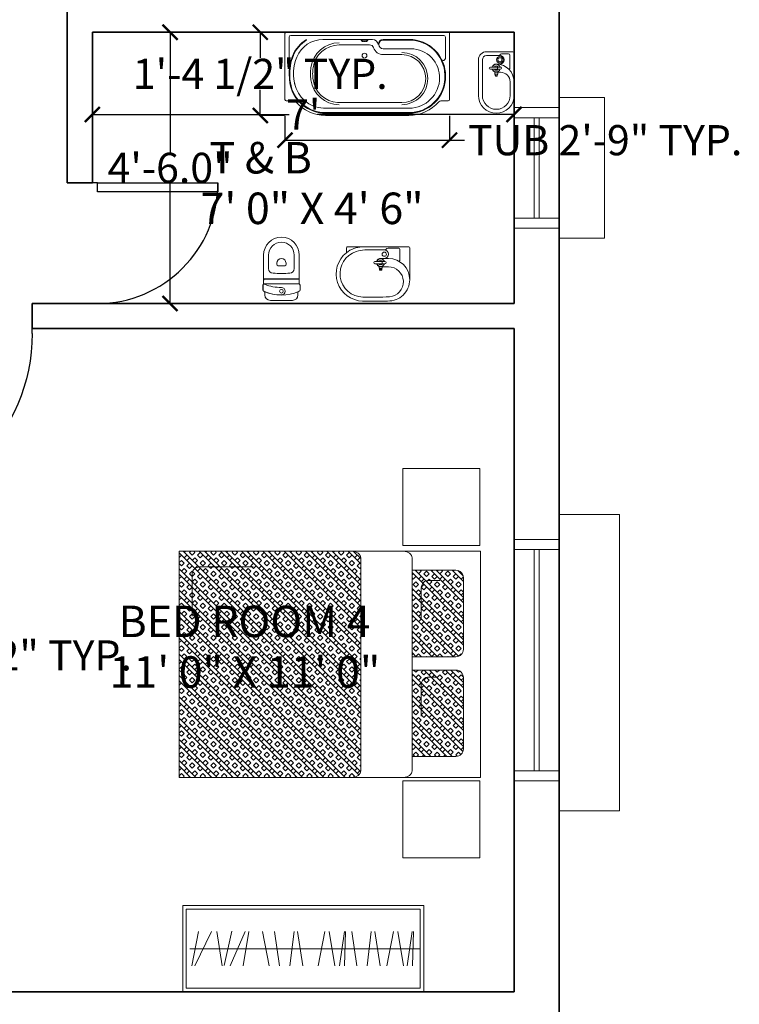
# Model space of a CAD drawing. Units: inches. Extents: x 844 to 2234, y 346 to 1084.
# Tile 91 of 93: x 2069 to 2212, y 632 to 828. Entities that reach past the tile are written whole.
import ezdxf

# ---------------------------------------------------------------- set-up
doc = ezdxf.new("R2010")
doc.units = ezdxf.units.IN
doc.header["$MEASUREMENT"] = 0
for name, color, linetype, lineweight in [('A-ANNO-DIMS', 2, 'Continuous', 18), ('A-AREA-IDEN', 7, 'Continuous', 18), ('A-FLOR-FIXT', 8, 'Continuous', 18), ('A-WALL', 7, 'Continuous', 35), ('beds', 130, 'Continuous', 18), ('doors', 170, 'Continuous', 25), ('furniture', 8, 'Continuous', 18), ('windows', 1, 'Continuous', 18)]:
    doc.layers.add(name, color=color, linetype=linetype, lineweight=lineweight)
doc.styles.get("Standard").update_dxf_attribs({"font": 'arial.ttf'})
doc.dimstyles.get("Standard").update_dxf_attribs({"dimtxt": 6, "dimasz": 3, "dimexe": 0.18, "dimexo": 0.0625, "dimgap": 0.09, "dimtad": 0, "dimtih": 1, "dimtoh": 1, "dimdec": 1, "dimzin": 0, "dimdsep": 46, "dimlunit": 3, "dimtxsty": 'Standard', "dimblk": 'ARCHTICK', "dimcen": 0.09, "dimadec": 0, "dimazin": 0, "dimtfac": 1, "dimtdec": 1, "dimtofl": 0, "dimtmove": 0, "dimatfit": 3, "dimfxl": 1, "dimtolj": 1, "dimtzin": 0, "dimarcsym": 0})
pattern_1 = [(135, (-1377.70473, -125.71507), (-0.070710678, -0.070710678), []), (135, (-1377.68705, -125.69739), (-0.070710678, -0.070710678), []), (45, (-1377.70473, -125.71507), (-0.070710678, 0.070710678), [-0.025, 0.025]), (45, (-1377.72241, -125.69739), (-0.070710678, 0.070710678), [-0.025, 0.025]), (45, (-1377.74009, -125.67972), (-0.070710678, 0.070710678), [0.025, -0.025]), (45, (-1377.75776, -125.66204), (-0.070710678, 0.070710678), [0.025, -0.025]), (135, (-1377.66938, -125.67972), (-0.070710678, -0.070710678), [0.025, -0.025]), (135, (-1377.6517, -125.66204), (-0.070710678, -0.070710678), [0.025, -0.025])]

# ---------------------------------------------------------------- blocks, each defined once
blk = doc.blocks.new('*U2')
for p, q in [((0, 0), (0, -6)), ((36, 0), (36, -6))]:
    blk.add_line(p, q)
blk.add_lwpolyline([(0, 0), (0, 36), (1.75, 36), (1.75, 0)], close=True)
blk.add_arc((0, 0), 36, 0, 90)
blk = doc.blocks.new('*U4')
for p, q in [((0, 0), (0, -6)), ((24, 0), (24, -6))]:
    blk.add_line(p, q)
blk.add_lwpolyline([(0, 0), (0, 24), (1.75, 24), (1.75, 0)], close=True)
blk.add_arc((0, 0), 24, 0, 90)
blk = doc.blocks.new('MAT-P10')
h = blk.add_hatch()
h.set_pattern_fill('BOX', color=256, scale=0.1, angle=45, style=0)
h.set_pattern_definition(pattern_1)
h.paths.add_polyline_path([(-0.1565, 1.4605), (0.417, 1.4605), (0.417, 1.7513, 0.414214), (0.367, 1.8013), (-0.1065, 1.8013, 0.414214), (-0.1565, 1.7513)])
h.paths.add_polyline_path([(0.5052, 1.4604), (1.0792, 1.4604), (1.0792, 1.7513, 0.414214), (1.0292, 1.8013), (0.5552, 1.8013, 0.414214), (0.5052, 1.7513)])
h = blk.add_hatch()
h.set_pattern_fill('BOX', color=256, scale=0.1, angle=45, style=0)
h.set_pattern_definition(pattern_1)
edge = h.paths.add_edge_path()
edge.add_line((1.2049, -0.085), (1.2049, 1.0625))
edge.add_ellipse((1.1608, 1.0627), major_axis=(0, 0.0568), ratio=0.776379, start_angle=270, end_angle=360)
edge.add_line((1.1608, 1.1195), (-0.251, 1.1195))
edge.add_ellipse((-0.251, 1.0627), major_axis=(0, 0.0568), ratio=0.776379, start_angle=0, end_angle=88.13958)
edge.add_line((-0.2951, 1.0641), (-0.2951, -0.085))
edge.add_line((-0.2951, -0.085), (1.2049, -0.085))
for p, q in [((-0.251, 1.4605), (1.1608, 1.4604)), ((-0.251, 1.1195), (1.1608, 1.1195)), ((1.1017, 0.406), (1.1017, 0.0572)), ((1.0576, 0.0004), (0.7754, 0.0004))]:
    blk.add_line(p, q)
for points in [[(-0.8301, 1.9091), (-0.3191, 1.9091), (-0.3191, 1.3981), (-0.8301, 1.3981)], [(1.2049, -0.085), (-0.2951, -0.085), (-0.2951, 1.9151), (1.2049, 1.915)], [(1.2441, 1.9091), (1.755, 1.9091), (1.755, 1.3981), (1.2441, 1.3981)]]:
    blk.add_lwpolyline(points, close=True)
for points in [[(0.417, 1.4604), (0.417, 1.7513, 0.414214), (0.367, 1.8013), (-0.1065, 1.8013, 0.414214), (-0.1565, 1.7513), (-0.1565, 1.4604)], [(1.0792, 1.4603), (1.0792, 1.7513, 0.414214), (1.0292, 1.8013), (0.5552, 1.8013, 0.414214), (0.5052, 1.7513), (0.5052, 1.4604)], [(1.0117, 1.6438), (1.0117, 1.5715, -0.414214), (0.9617, 1.5215), (0.7528, 1.5215)], [(0.3702, 1.6242), (0.3702, 1.5715, -0.414214), (0.3202, 1.5215), (0.1113, 1.5215)]]:
    blk.add_lwpolyline(points, format="xyb")
at = {"extrusion": (0, 0, -1)}
for centre, start_param, end_param in [((-0.251, 1.4036), 4.712389, 6.283185), ((1.1608, 1.4036), 0, 1.570796), ((-0.251, 1.0627), 4.712389, 6.283185), ((1.1608, 1.0627), 0, 1.570796), ((1.0576, 0.0572), 1.570796, 3.141593), ((1.0576, 0.0572), 1.570796, 3.141593)]:
    blk.add_ellipse(centre, major_axis=(0, 0.0568), ratio=0.776379, start_param=start_param, end_param=end_param, dxfattribs=at)
blk = doc.blocks.new('A$C7A17768A')
for p, q in [((-2.8, 0), (0, 0)), ((-2.8, -1), (-2.8, 0)), ((0, -1), (0, 0)), ((-2.76, -0.04), (-0.04, -0.04)), ((-2.76, -0.96), (-2.76, -0.04)), ((-0.04, -0.96), (-0.04, -0.04)), ((-2.617, -0.3), (-2.694, -0.7)), ((-2.66, -0.7), (-2.466, -0.3)), ((-2.403, -0.3), (-2.342, -0.7)), ((-2.229, -0.296), (-2.317, -0.696)), ((-2.074, -0.3), (-2.25, -0.7)), ((-2.096, -0.7), (-2.033, -0.3)), ((-1.875, -0.3), (-1.796, -0.7)), ((-1.732, -0.3), (-1.675, -0.7)), ((-1.555, -0.7), (-1.507, -0.3)), ((-1.467, -0.3), (-1.403, -0.7)), ((-1.227, -0.7), (-1.151, -0.3)), ((-1.098, -0.3), (-1.034, -0.7)), ((-0.98, -0.7), (-0.921, -0.3)), ((-0.908, -0.3), (-0.919, -0.7)), ((-0.834, -0.3), (-0.777, -0.7)), ((-0.657, -0.7), (-0.61, -0.3)), ((-0.57, -0.3), (-0.505, -0.7)), ((-0.429, -0.7), (-0.353, -0.3)), ((-0.301, -0.3), (-0.237, -0.7)), ((-0.192, -0.7), (-0.133, -0.3)), ((-0.12, -0.3), (-0.131, -0.7)), ((-0.04, -0.5), (-2.716, -0.5)), ((-2.8, -1), (0, -1)), ((-2.76, -0.96), (-0.04, -0.96))]:
    blk.add_line(p, q)
blk = doc.blocks.new('2SABICO')
at = {"color": 0, "linetype": 'ByBlock'}
for p, q in [((0.478, 0.195), (0.089, 0.195)), ((0.478, 0.152), (0.089, 0.152)), ((0, 0.106), (0, 0)), ((0, 0), (0, -0.18)), ((0.043, -0.039), (0.043, 0.106)), ((0.135, 0), (0.135, -0.003)), ((0.168, 0.064), (0.168, -0.015)), ((0.192, 0.064), (0.192, -0.015)), ((0.221, 0.012), (0.222, 0.012)), ((0.223, 0.016), (0.223, -0.016)), ((0.224, 0.017), (0.245, 0.017)), ((0.246, 0.016), (0.246, -0.016)), ((0.25, 0.014), (0.246, 0.014)), ((0.26, 0.01), (0.268, 0.01)), ((0.268, -0.01), (0.268, 0.01)), ((0.268, 0.01), (0.269, 0.009)), ((0.269, -0.009), (0.269, 0.009)), ((0.023, -0.057), (0.023, -0.135)), ((0.135, 0), (0.135, -0.039)), ((0.168, -0.015), (0.192, -0.015)), ((0.168, -0.015), (0.168, -0.046)), ((0.192, -0.015), (0.192, -0.046)), ((0.221, -0.012), (0.222, -0.012)), ((0.224, -0.017), (0.245, -0.017)), ((0.225, -0.017), (0.225, -0.047)), ((0.25, -0.014), (0.246, -0.014)), ((0.26, -0.01), (0.268, -0.01)), ((0.268, -0.01), (0.269, -0.009)), ((0.015, -0.195), (0.478, -0.195)), ((0.038, -0.15), (0.179, -0.15)), ((0.33, -0.152), (0.478, -0.152))]:
    blk.add_line(p, q, dxfattribs=at)
for radius in [0.035, 0.023]:
    blk.add_circle((0.089, -0.039), radius, dxfattribs=at)
for centre, radius, start, end in [((0.089, 0.106), 0.089, 90, 180), ((0.089, 0.106), 0.046, 90, 180), ((0.478, 0), 0.195, 270, 90), ((0.478, 0), 0.152, 270, 90), ((0.18, 0), 0.045, 105.6643, 180), ((0.18, 0), 0.042, 106.8152, 252.6853), ((0.18, 0), 0.0235, 121.1327, 237.8651), ((0.18, 0.064), 0.0121, 0, 180), ((0.18, 0), 0.045, 17.0576, 74.3357), ((0.18, 0), 0.042, 287.3147, 73.1848), ((0.18, 0), 0.0235, 302.1349, 58.8673), ((0.221, 0.013), 0.001, 197.9471, 270), ((0.222, 0.013), 0.001, 270, 0), ((0.224, 0.016), 0.001, 90, 180), ((0.245, 0.016), 0.001, 0, 90), ((0.25, 0), 0.0143, 270, 90), ((0.041, -0.057), 0.018, 99.5941, 180), ((0.037, -0.033), 0.006, 279.5941, 0), ((0.089, -0.039), 0.046, 180, 360), ((0.326, -0.003), 0.191, 180, 270), ((0.18, -0.046), 0.0125, 180, 0), ((0.221, -0.013), 0.001, 90, 162.0529), ((0.222, -0.013), 0.001, 0, 90), ((0.224, -0.016), 0.001, 180, 270), ((0.33, -0.047), 0.105, 180, 270), ((0.245, -0.016), 0.001, 270, 0), ((0.015, -0.18), 0.015, 180, 270), ((0.038, -0.135), 0.015, 180, 270), ((0.179, -0.14), 0.01, 270, 42.9682)]:
    blk.add_arc(centre, radius, start, end, dxfattribs=at)
blk = doc.blocks.new('2SAINCO')
at = {"color": 0, "linetype": 'ByBlock'}
for p, q in [((0, -0.121), (0, 0.121)), ((0.06, 0.181), (0.085, 0.181)), ((0.114, 0.203), (0.165, 0.203)), ((0.496, 0.195), (0.178, 0.195)), ((0.18, -0.188), (0.18, 0.188)), ((0.231, 0.185), (0.231, -0.185)), ((0.234, 0.185), (0.234, -0.185)), ((0.496, 0.14), (0.347, 0.14)), ((0.394, 0.05), (0.407, 0.05)), ((0.394, -0.05), (0.407, -0.05)), ((0.06, -0.181), (0.085, -0.181)), ((0.114, -0.201), (0.165, -0.201)), ((0.114, -0.203), (0.165, -0.203)), ((0.496, -0.195), (0.178, -0.195)), ((0.496, -0.14), (0.347, -0.14))]:
    blk.add_line(p, q, dxfattribs=at)
blk.add_circle((0.1, 0), 0.02, dxfattribs=at)
for centre, radius, start, end in [((0.06, 0.121), 0.06, 90, 180), ((0.517, 0), 0.46, 155.909, 204.091), ((0.085, 0.196), 0.015, 270, 344.534), ((0.114, 0.188), 0.015, 90, 164.534), ((0.165, 0.188), 0.015, 0, 90), ((0.221, 0.185), 0.01, 0, 90), ((0.224, 0.185), 0.01, 0, 90), ((0.347, 0.09), 0.05, 90, 177.3546), ((0.496, 0), 0.195, 270, 90), ((0.496, 0), 0.14, 270, 90), ((0.1, 0), 0.0405, 360, 180), ((0.517, 0), 0.458, 180, 204.67), ((0.66, 0.008), 0.52, 180.891, 201.3823), ((2.295, 0), 2, 177.3546, 182.6454), ((0.677, 0), 0.3, 172.9459, 187.0541), ((0.394, 0.035), 0.015, 90, 172.9459), ((0.407, 0), 0.05, 270, 90), ((0.347, -0.09), 0.05, 182.6454, 270), ((0.394, -0.035), 0.015, 187.0541, 270), ((0.06, -0.121), 0.06, 180, 270), ((0.085, -0.196), 0.015, 15.466, 90), ((0.114, -0.188), 0.015, 195.466, 270), ((0.114, -0.188), 0.013, 195.466, 270), ((0.165, -0.188), 0.013, 270, 30), ((0.165, -0.188), 0.015, 270, 0), ((0.221, -0.185), 0.01, 270, 0), ((0.224, -0.185), 0.01, 270, 0)]:
    blk.add_arc(centre, radius, start, end, dxfattribs=at)
blk = doc.blocks.new('2SABACO')
at = {"color": 0}
for p, q in [((1.341, 0.91), (0.429, 0.91)), ((1.341, 0.885), (0.429, 0.885)), ((1.341, 0.879), (0.429, 0.879)), ((1.341, 0.831), (0.407, 0.831)), ((1.263, 0.769), (0.562, 0.769)), ((-0.015, 0.735), (-0.015, 0.015)), ((0, 0.75), (0.08, 0.75)), ((1.77, 0.75), (1.69, 0.75)), ((1.785, 0.015), (1.785, 0.735)), ((0.03, 0.302), (0.03, 0.053)), ((1.263, 0.245), (1.06, 0.245)), ((1.74, 0.053), (1.74, 0.286)), ((0.578, 0.139), (0.911, 0.139)), ((1.363, 0.181), (1.06, 0.181)), ((0, 0), (1.77, 0)), ((0.048, 0.035), (1.722, 0.035)), ((0.401, 0.08), (0.942, 0.08)), ((1.343, 0.086), (1.06, 0.086)), ((1.343, 0.079), (1.06, 0.079))]:
    blk.add_line(p, q, dxfattribs=at)
blk.add_circle((0.855, 0.256), 0.026, dxfattribs=at)
for centre, radius, start, end in [((0.428, 0.49), 0.395, 98.9726, 181.1954), ((0.428, 0.49), 0.389, 98.9726, 181.2301), ((0.429, 0.48), 0.43, 90, 139.2943), ((0.429, 0.48), 0.405, 90, 98.9726), ((0.429, 0.48), 0.399, 90, 98.9726), ((1.341, 0.48), 0.43, 40.7057, 90), ((1.341, 0.485), 0.401, 359.4627, 90), ((1.341, 0.485), 0.394, 3.5237, 90), ((0.08, 0.78), 0.03, 270, 319.2943), ((0.425, 0.49), 0.342, 93.1008, 168.0202), ((0.578, 0.481), 0.311, 90, 172.609), ((0.578, 0.481), 0.288, 93.3767, 172.609), ((1.263, 0.507), 0.285, 270, 90), ((1.263, 0.507), 0.262, 270, 90), ((1.341, 0.495), 0.336, 0, 90), ((1.69, 0.78), 0.03, 220.7057, 270), ((0, 0.735), 0.015, 90, 180), ((1.77, 0.735), 0.015, 0, 90), ((0.559, 0.454), 0.48, 163.1286, 202.3619), ((0.559, 0.454), 0.528, 177.0415, 202.3619), ((0.559, 0.454), 0.521, 177.0156, 202.3619), ((0.79, 0.454), 0.525, 172.609, 180), ((0.79, 0.454), 0.525, 180, 187.391), ((0.79, 0.454), 0.502, 172.609, 180), ((0.79, 0.454), 0.502, 180, 187.391), ((1.343, 0.477), 0.392, 270, 4.5675), ((1.343, 0.477), 0.398, 270, 0.539), ((1.363, 0.495), 0.314, 270, 2.2815), ((0.578, 0.427), 0.311, 187.391, 270), ((0.578, 0.427), 0.288, 187.391, 270), ((0.042, 0.302), 0.0116, 16.3184, 180.0001), ((0.401, 0.389), 0.357, 202.3619, 239.8287), ((0.401, 0.389), 0.351, 202.3619, 239.2093), ((0.401, 0.389), 0.309, 202.3619, 270), ((1.06, 0.133), 0.112, 90, 161.2369), ((1.718, 0.286), 0.0222, 0, 152.9966), ((0.911, 0.183), 0.045, 270, 341.2369), ((0.942, 0.145), 0.065, 270, 349.4977), ((1.06, 0.133), 0.054, 180, 270), ((1.06, 0.133), 0.0475, 90, 270), ((0, 0.015), 0.015, 180, 270), ((0.048, 0.053), 0.018, 180, 270), ((0.559, 0.454), 0.48, 250.7818, 251.0555), ((0.821, 0.092), 0.00282, 119.7759, 180), ((0.821, 0.092), 0.00282, 180, 240.2241), ((0.837, 0.064), 0.0347, 103.3326, 119.7759), ((0.835, 0.025), 0.071, 96.5949, 102.1924), ((0.837, 0.12), 0.0347, 240.2241, 256.6674), ((0.847, -0.08), 0.177, 92.7417, 96.5949), ((0.848, 0.02), 0.0808, 95.6065, 103.3326), ((0.848, 0.164), 0.0808, 256.6674, 264.3935), ((0.855, -0.252), 0.349, 90, 92.7417), ((0.855, -0.053), 0.153, 90, 95.6065), ((0.855, 0.237), 0.153, 264.3935, 270), ((0.855, -0.053), 0.153, 84.3935, 90), ((0.855, -0.252), 0.349, 87.2583, 90), ((0.855, 0.237), 0.153, 270, 275.6065), ((0.862, 0.02), 0.0808, 76.6674, 84.3935), ((0.862, 0.164), 0.0808, 275.6065, 283.3326), ((0.863, -0.08), 0.177, 83.4051, 87.2583), ((0.873, 0.064), 0.0347, 60.2241, 76.6674), ((0.873, 0.12), 0.0347, 283.3326, 299.7759), ((0.875, 0.025), 0.071, 77.8076, 83.4051), ((0.889, 0.092), 0.00282, 360, 60.2241), ((0.889, 0.092), 0.00282, 299.7759, 360), ((1.722, 0.053), 0.018, 270, 0), ((1.77, 0.015), 0.015, 270, 0)]:
    blk.add_arc(centre, radius, start, end, dxfattribs=at)
blk = doc.blocks.new('2SALACO2')
at = {"color": 0}
for p, q in [((0, 0), (-0.392, 0)), ((0.28, 0), (0, 0)), ((-0.402, -0.01), (-0.402, -0.36)), ((-0.293, -0.026), (-0.293, -0.15)), ((-0.283, -0.016), (-0.166, -0.016)), ((-0.112, -0.035), (-0.133, -0.035)), ((-0.124, -0.035), (0.09, -0.035)), ((0.29, -0.01), (0.29, -0.064)), ((-0.169, -0.128), (-0.085, -0.128)), ((-0.1, -0.161), (-0.131, -0.161)), ((-0.1, -0.186), (-0.131, -0.186)), ((-0.1, -0.161), (-0.1, -0.186)), ((-0.021, -0.161), (-0.1, -0.161)), ((-0.021, -0.186), (-0.1, -0.186)), ((-0.098, -0.214), (-0.098, -0.216)), ((-0.073, -0.214), (-0.073, -0.216)), ((-0.102, -0.219), (-0.169, -0.219)), ((-0.102, -0.217), (-0.102, -0.234)), ((-0.07, -0.216), (-0.101, -0.216)), ((-0.07, -0.235), (-0.101, -0.235)), ((-0.097, -0.239), (-0.098, -0.241)), ((-0.098, -0.241), (-0.098, -0.248)), ((-0.098, -0.241), (-0.073, -0.241)), ((-0.073, -0.248), (-0.098, -0.248)), ((-0.097, -0.235), (-0.097, -0.239)), ((-0.074, -0.239), (-0.097, -0.239)), ((-0.097, -0.248), (-0.097, -0.256)), ((-0.073, -0.256), (-0.097, -0.256)), ((-0.097, -0.256), (-0.094, -0.257)), ((-0.077, -0.257), (-0.094, -0.257)), ((-0.073, -0.256), (-0.077, -0.257)), ((-0.074, -0.235), (-0.074, -0.239)), ((-0.074, -0.239), (-0.073, -0.241)), ((-0.073, -0.241), (-0.073, -0.248)), ((-0.073, -0.248), (-0.073, -0.256)), ((-0.069, -0.217), (-0.069, -0.234))]:
    blk.add_line(p, q, dxfattribs=at)
blk.add_lwpolyline([(-0.402, -0.36, 0.423787), (-0.161, -0.593, 0.423787)], format="xyb", dxfattribs=at)
blk.add_circle((-0.124, -0.081), 0.023, dxfattribs=at)
for centre, radius, start, end in [((-0.392, -0.01), 0.01, 90, 180), ((0.28, -0.01), 0.01, 0, 90), ((-0.283, -0.026), 0.01, 90, 180), ((-0.124, -0.081), 0.0462, 90, 270), ((-0.166, -0.046), 0.03, 31.2573, 90), ((-0.133, -0.026), 0.009, 211.2573, 270), ((0.09, -0.29), 0.255, 68.9449, 90), ((0.105, -0.295), 0.255, 271.0077, 72.4499), ((0.105, -0.297), 0.297, 271.4871, 51.4524), ((0.105, -0.297), 0.297, 51.4524, 87.1707), ((-0.169, -0.36), 0.233, 90, 180), ((-0.285, -0.15), 0.008, 180, 299.1062), ((-0.131, -0.173), 0.0125, 90, 270), ((-0.085, -0.173), 0.042, 16.8152, 162.6853), ((-0.085, -0.173), 0.042, 197.3147, 343.1848), ((-0.085, -0.173), 0.0235, 31.1327, 147.8651), ((-0.085, -0.173), 0.0235, 212.1349, 328.8673), ((-0.085, -0.173), 0.0458, 15.3964, 90), ((-0.085, -0.173), 0.0458, 289.9182, 344.6036), ((-0.021, -0.173), 0.0121, 270, 90), ((-0.169, -0.383), 0.164, 90, 265.4963), ((-0.101, -0.217), 0.001, 90, 180), ((-0.101, -0.234), 0.001, 180, 270), ((-0.07, -0.217), 0.001, 0, 90), ((-0.07, -0.234), 0.001, 270, 0), ((0.021, 4.449), 5, 267.6742, 271.0081), ((-0.017, 4.405), 5, 268.3511, 271.4874)]:
    blk.add_arc(centre, radius, start, end, dxfattribs=at)
blk = doc.blocks.new('_ArchTick')
at = {"color": 0, "linetype": 'ByBlock', "const_width": 0.15}
blk.add_lwpolyline([(-0.5, -0.5), (0.5, 0.5)], dxfattribs=at)
blk = doc.blocks.new('*D72')
at = {"layer": 'A-ANNO-DIMS', "color": 0, "lineweight": -2, "transparency": 16777216}
for p, q in [((2109.21, 825.46), (2098.4, 825.46)), ((2098.58, 825.46), (2098.58, 801.61)), ((2098.58, 771.46), (2098.58, 795.3)), ((2109.21, 771.46), (2098.4, 771.46))]:
    blk.add_line(p, q, dxfattribs=at)
at = {"layer": 'Defpoints', "color": 0, "transparency": 16777216}
for p in [(2109.27, 825.46), (2098.58, 771.46), (2109.27, 771.46)]:
    blk.add_point(p, dxfattribs=at)
at = {"layer": 'A-ANNO-DIMS', "color": 0, "lineweight": -2, "transparency": 16777216, "xscale": 3, "yscale": 3, "zscale": 3}
for p, rotation in [((2098.58, 825.46), 90), ((2098.58, 771.46), 270)]:
    blk.add_blockref('_ArchTick', p, dxfattribs=dict(at, rotation=rotation))
at = {"layer": 'A-ANNO-DIMS', "color": 0, "transparency": 16777216, "insert": (2098.58, 798.46), "char_height": 6, "attachment_point": 5}
blk.add_mtext('\\A1;4\'-6.0"', dxfattribs=at)
blk = doc.blocks.new('*D73')
at = {"layer": 'A-ANNO-DIMS', "color": 0, "lineweight": -2, "transparency": 16777216}
for p, q in [((2083.1, 809.15), (2083.1, 809.27)), ((2083.1, 809.09), (2122.27, 809.09)), ((2167.1, 809.09), (2127.93, 809.09)), ((2167.1, 809.15), (2167.1, 809.27))]:
    blk.add_line(p, q, dxfattribs=at)
at = {"layer": 'Defpoints', "color": 0, "transparency": 16777216}
for p in [(2083.1, 809.09), (2083.1, 809.09), (2167.1, 809.09)]:
    blk.add_point(p, dxfattribs=at)
at = {"layer": 'A-ANNO-DIMS', "color": 0, "lineweight": -2, "transparency": 16777216, "xscale": 3, "yscale": 3, "zscale": 3, "rotation": 180}
blk.add_blockref('_ArchTick', (2083.1, 809.09), dxfattribs=at)
at = {"layer": 'A-ANNO-DIMS', "color": 0, "lineweight": -2, "transparency": 16777216, "xscale": 3, "yscale": 3, "zscale": 3}
blk.add_blockref('_ArchTick', (2167.1, 809.09), dxfattribs=at)
at = {"layer": 'A-ANNO-DIMS', "color": 0, "transparency": 16777216, "insert": (2125.1, 809.09), "char_height": 6, "attachment_point": 5}
blk.add_mtext("\\A1;7'", dxfattribs=at)
blk = doc.blocks.new('WIN-48IN')
for p, q in [((0, 9), (0, 21)), ((0, 21), (59, 21)), ((59, 9), (59, 21)), ((6, 9), (0, 9)), ((54, 9), (6, 9)), ((6, 9), (6, 0)), ((8, 9), (8, 0)), ((52, 0), (52, 9)), ((54, 0), (54, 9)), ((54, 9), (59, 9)), ((8, 5), (52, 5)), ((8, 4), (52, 4)), ((6, 0), (54, 0))]:
    blk.add_line(p, q)
blk = doc.blocks.new('WIN-24IN')
for p, q in [((9, 28), (0, 28)), ((0, 0), (0, 28)), ((9, 26), (9, 28)), ((18, 26), (9, 26)), ((9, 26), (9, 2)), ((18, 2), (18, 26)), ((18, 24), (9, 24)), ((13, 4), (13, 24)), ((14, 4), (14, 24)), ((9, 4), (18, 4)), ((9, 2), (18, 2)), ((9, 2), (9, 0)), ((9, 0), (0, 0))]:
    blk.add_line(p, q)
blk = doc.blocks.new('*D115')
at = {"layer": 'A-ANNO-DIMS', "color": 0, "lineweight": -2, "transparency": 16777216}
for p, q in [((2121.46, 808.82), (2121.46, 803.79)), ((2154.24, 808.82), (2154.24, 803.79)), ((2121.46, 803.97), (2154.24, 803.97)), ((2154.24, 803.97), (2157.24, 803.97))]:
    blk.add_line(p, q, dxfattribs=at)
at = {"layer": 'Defpoints', "color": 0, "transparency": 16777216}
for p in [(2121.46, 808.88), (2154.24, 808.88), (2154.24, 803.97)]:
    blk.add_point(p, dxfattribs=at)
at = {"layer": 'A-ANNO-DIMS', "color": 0, "lineweight": -2, "transparency": 16777216, "xscale": 3, "yscale": 3, "zscale": 3, "rotation": 180}
blk.add_blockref('_ArchTick', (2121.46, 803.97), dxfattribs=at)
at = {"layer": 'A-ANNO-DIMS', "color": 0, "lineweight": -2, "transparency": 16777216, "xscale": 3, "yscale": 3, "zscale": 3}
blk.add_blockref('_ArchTick', (2154.24, 803.97), dxfattribs=at)
at = {"layer": 'A-ANNO-DIMS', "color": 0, "transparency": 16777216, "insert": (2185.24, 803.97), "char_height": 6, "attachment_point": 5}
blk.add_mtext('\\A1;TUB 2\'-9" TYP.', dxfattribs=at)
blk = doc.blocks.new('*D116')
at = {"layer": 'A-ANNO-DIMS', "color": 0, "lineweight": -2, "transparency": 16777216}
for p, q in [((2121.39, 825.46), (2116.36, 825.46)), ((2116.54, 825.46), (2116.54, 820.36)), ((2116.54, 808.88), (2116.54, 813.98)), ((2121.39, 808.88), (2116.36, 808.88))]:
    blk.add_line(p, q, dxfattribs=at)
at = {"layer": 'Defpoints', "color": 0, "transparency": 16777216}
for p in [(2121.46, 825.46), (2116.54, 808.88), (2121.46, 808.88)]:
    blk.add_point(p, dxfattribs=at)
at = {"layer": 'A-ANNO-DIMS', "color": 0, "lineweight": -2, "transparency": 16777216, "xscale": 3, "yscale": 3, "zscale": 3}
for p, rotation in [((2116.54, 825.46), 90), ((2116.54, 808.88), 270)]:
    blk.add_blockref('_ArchTick', p, dxfattribs=dict(at, rotation=rotation))
at = {"layer": 'A-ANNO-DIMS', "color": 0, "transparency": 16777216, "insert": (2116.54, 817.17), "char_height": 6, "attachment_point": 5}
blk.add_mtext('\\A1;1\'-4 1/2" TYP.', dxfattribs=at)
blk = doc.blocks.new('*D121')
at = {"layer": 'A-ANNO-DIMS', "color": 0, "lineweight": -2, "transparency": 16777216}
for p, q in [((2030.27, 734.26), (2040.25, 734.26)), ((2040.07, 734.26), (2040.07, 704.6)), ((2040.07, 668.56), (2040.07, 698.22)), ((2030.27, 668.56), (2040.25, 668.56))]:
    blk.add_line(p, q, dxfattribs=at)
at = {"layer": 'Defpoints', "color": 0, "transparency": 16777216}
for p in [(2030.21, 734.26), (2040.07, 734.26), (2030.21, 668.56)]:
    blk.add_point(p, dxfattribs=at)
at = {"layer": 'A-ANNO-DIMS', "color": 0, "lineweight": -2, "transparency": 16777216, "xscale": 3, "yscale": 3, "zscale": 3}
for p, rotation in [((2040.07, 734.26), 90), ((2040.07, 668.56), 270)]:
    blk.add_blockref('_ArchTick', p, dxfattribs=dict(at, rotation=rotation))
at = {"layer": 'A-ANNO-DIMS', "color": 0, "transparency": 16777216, "insert": (2040.07, 701.41), "char_height": 6, "attachment_point": 5}
blk.add_mtext('\\A1;LOUNGE SET 5\'-5 1/2" TYP.', dxfattribs=at)

msp = doc.modelspace()

# ---------------------------------------------------------------- linework, layer by layer
at = {"layer": 'A-WALL'}
for p, q in [((2176.1, 1030.46), (2176.1, 435.46)), ((2078.1, 884.46), (2078.1, 795.46)), ((2083.1, 825.46), (2083.1, 795.46)), ((2167.1, 825.46), (2083.1, 825.46)), ((2167.1, 825.46), (2167.1, 771.46)), ((2078.1, 795.46), (2083.1, 795.46)), ((2078.1, 771.46), (2071.1, 771.46)), ((2071.1, 766.46), (2071.1, 771.46)), ((2078.1, 771.46), (2083.1, 771.46)), ((2167.1, 771.46), (2083.1, 771.46)), ((2167.1, 766.46), (2071.1, 766.46)), ((2167.1, 766.46), (2167.1, 634.46)), ((2167.1, 634.46), (2035.1, 634.46))]:
    msp.add_line(p, q, dxfattribs=at)

# ---------------------------------------------------------------- block references
at = {"layer": 'A-FLOR-FIXT', "xscale": -18.21101258924898, "yscale": 18.21101258924898, "zscale": 18.21101258924898}
for name, p, rotation in [('2SABACO', (2121.73, 825.46), 180), ('2SABICO', (2163.55, 821.59), 90), ('2SAINCO', (2120.76, 772.08), 270)]:
    msp.add_blockref(name, p, dxfattribs=dict(at, rotation=rotation))
msp.add_blockref('2SALACO2', (2138.98, 782.75), dxfattribs=at)
at = {"layer": 'beds', "xscale": -29.99962925113936, "yscale": 29.99962925113936, "zscale": 29.99962925113936, "rotation": 270}
msp.add_blockref('MAT-P10', (2102.97, 685.99), dxfattribs=at)
at = {"layer": 'doors', "rotation": 270}
msp.add_blockref('*U4', (2084.1, 795.46), dxfattribs=at)
at = {"layer": 'doors', "xscale": -1, "rotation": 180}
msp.add_blockref('*U2', (2035.1, 765.46), dxfattribs=at)
at = {"layer": 'furniture', "xscale": 17.14285714285603, "yscale": 17.14285714285603, "zscale": 17.14285714285603}
msp.add_blockref('A$C7A17768A', (2149.1, 651.6), dxfattribs=at)
at = {"layer": 'windows', "rotation": 180}
msp.add_blockref('WIN-24IN', (2185.1, 812.45), dxfattribs=at)
at = {"layer": 'windows', "extrusion": (0, 0, -1), "zscale": -1, "rotation": 90.0000000000031}
msp.add_blockref('WIN-48IN', (-2167.1, 670.46), dxfattribs=at)

# ---------------------------------------------------------------- texts
at = {"layer": 'A-AREA-IDEN'}
for s, height, p in [('T & B', 6.269, (2106.43, 797.34)), (' 7\' 0" X 4\' 6"', 6.2688, (2102.73, 787.27)), ('BED ROOM 4', 6.269, (2088.31, 705.04)), (' 11\' 0" X 11\' 0"', 6.2688, (2084.62, 694.97))]:
    msp.add_text(s, height=height, dxfattribs=at).set_placement(p)

# ---------------------------------------------------------------- dimensions: what is measured, and where the dimension line sits
at = {"layer": 'A-ANNO-DIMS'}
for base, p1, p2, angle, text, picture, middle in [((2116.54, 808.88), (2121.46, 825.46), (2121.46, 808.88), 270, '<> TYP.', '*D116', (2116.54, 817.17)), ((2040.07, 734.26), (2030.21, 668.56), (2030.21, 734.26), 90, 'LOUNGE SET <> TYP.', '*D121', (2040.07, 701.41))]:
    dim = msp.add_linear_dim(base=base, p1=p1, p2=p2, angle=angle, text=text, dimstyle='Standard', override={"dimdec": 1, "dimlfac": 1, "dimrnd": 0, "dimzin": 1, "dimdsep": 46, "dimlunit": 4, "dimfrac": 2}, dxfattribs=at)
    dim.commit()
    dim.dimension.update_dxf_attribs({"geometry": picture, "text_midpoint": middle})
dim = msp.add_linear_dim(base=(2098.58, 771.46), p1=(2109.27, 825.46), p2=(2109.27, 771.46), angle=90, dimstyle='Standard', override={"dimclrd": 0, "dimclre": 0, "dimclrt": 0}, dxfattribs=at)
dim.commit()
dim.dimension.update_dxf_attribs({"geometry": '*D72', "text_midpoint": (2098.58, 798.46)})
dim = msp.add_linear_dim(base=(2154.24, 803.97), p1=(2121.46, 808.88), p2=(2154.24, 808.88), text='TUB <> TYP.', dimstyle='Standard', override={"dimdec": 1, "dimlfac": 1, "dimrnd": 0, "dimzin": 1, "dimdsep": 46, "dimlunit": 4, "dimfrac": 2}, dxfattribs=at)
dim.commit()
dim.dimension.update_dxf_attribs({"geometry": '*D115', "text_midpoint": (2185.24, 803.97)})
dim = msp.add_linear_dim(base=(2083.1, 809.09), p1=(2167.1, 809.09), p2=(2083.1, 809.09), dimstyle='Standard', override={"dimclrd": 0, "dimclre": 0, "dimclrt": 0}, dxfattribs=at)
dim.commit()
dim.dimension.update_dxf_attribs({"geometry": '*D73', "text_midpoint": (2125.1, 809.09)})

doc.saveas('drawing.dxf')
